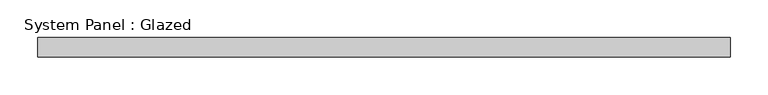
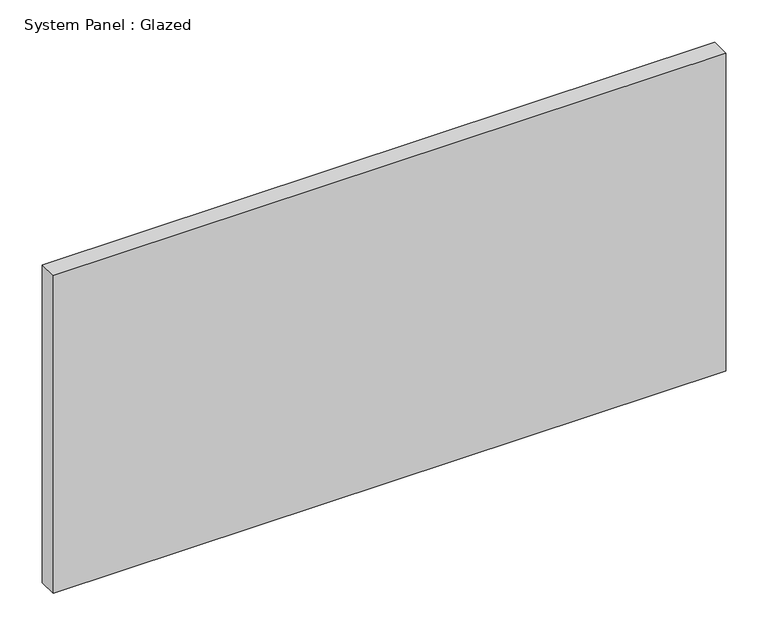
"""IFC4 building model written with IfcOpenShell, lengths in millimetres: plate geometry, System Panel : Glazed."""

from ifc_helpers import new_model, si_unit, origin, origin_with_axes, place, context, project, spatial, polyline, outline, extrude, source, transform, mapped, element, save


def system_panel_glazed_b74e51ee(model_context):
    return source(origin(), model_context, "Body", "SweptSolid", [
        extrude(outline(polyline([(457.1999998, -44.45), (-457.1999998, -44.45), (-457.1999998, -19.05), (457.1999998, -19.05), (457.1999998, -44.45)])), origin_with_axes(), (0.0, 0.0, 1.0), 457.2),
    ])


if __name__ == "__main__":
    model = new_model("IFC4")
    model_context = context("Model", 3, world=origin())
    ifc_project = project(units=[si_unit("LENGTHUNIT", "METRE", prefix="MILLI")], contexts=[model_context])
    site = spatial("IfcSite", under=ifc_project)
    building = spatial("IfcBuilding", under=site)
    placement = place(None, origin())
    system_panel_glazed_shape = system_panel_glazed_b74e51ee(model_context)
    element("IfcPlate", 1, ObjectType="System Panel : Glazed", at=placement, inside=building, context=model_context, shape_type="MappedRepresentation", body=[
        mapped(system_panel_glazed_shape, transform((0.0, 0.0, 0.0), x_axis=(1.0, 0.0, 0.0), y_axis=(0.0, 1.0, 0.0), z_axis=(0.0, 0.0, 1.0))),
    ])
    save(model, "model.ifc")

# Revit data of these elements
# Type "System Panel : Glazed"
#   Construction Type Id = "GSP4R"
#   Analytic Construction = "1/8 in Pilkington single glazing"
#   Visual Light Transmittance = 0.9
#   Solar Heat Gain Coefficient = 0.86
#   Heat Transfer Coefficient (U) = 1.18115 BTU/(h·ft²·°F)
#   Define Thermal Properties by = 1
# Element 1 (IfcPlate, "System Panel : Glazed")
#   Materials on its faces: "Glass"
# Materials
#   "Glass": class "Glass", colour RGB 0 128 192, transparency 0.75, Description = "Soda Lime Glass", Cost = 0
